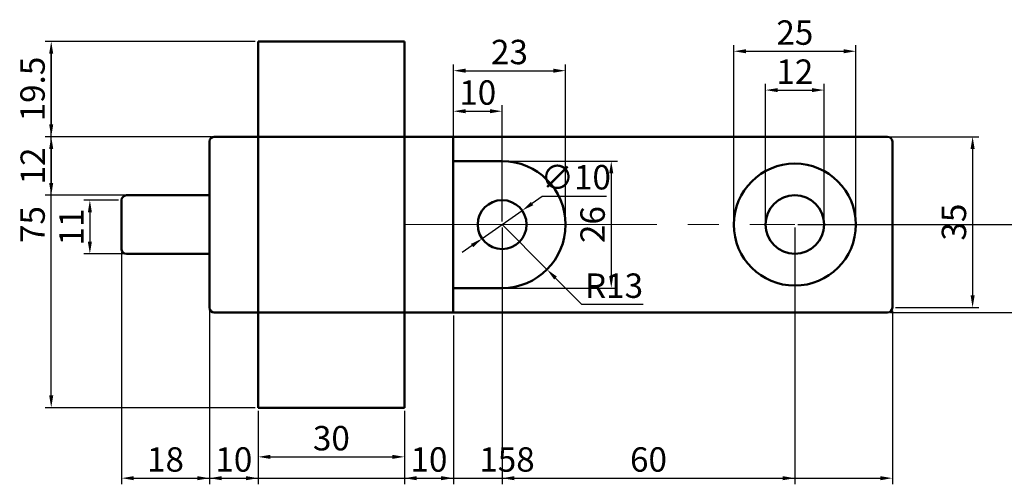
# Model space of a CAD drawing. Units: millimetres. Extents: x 2010 to 2347, y 1200 to 1429.
# Tile 1 of 3: x 2010 to 2212, y 1200 to 1295. Entities that reach past the tile are written whole.
import ezdxf

# ---------------------------------------------------------------- set-up
doc = ezdxf.new("R2010")
doc.units = ezdxf.units.MM
doc.linetypes.add('CENTER', pattern=[50.8, 31.75, -6.35, 6.35, -6.35])
for name, color, linetype, lineweight in [('M-CNTR', 4, 'CENTER', 18), ('M-DIMS', 2, 'Continuous', 25), ('M-OUTL', 7, 'Continuous', 50)]:
    doc.layers.add(name, color=color, linetype=linetype, lineweight=lineweight)
doc.styles.get("Standard").update_dxf_attribs({"font": 'arial.ttf'})
doc.dimstyles.new('ISO-25', dxfattribs={"dimtxt": 5, "dimasz": 2.5, "dimexe": 1.25, "dimexo": 0.625, "dimtad": 1, "dimtoh": 1, "dimdec": 0, "dimtxsty": 'Standard', "dimcen": 2.5, "dimadec": 0, "dimazin": 0, "dimtfac": 1, "dimtdec": 0, "dimtmove": 0, "dimatfit": 3, "dimfxl": 1, "dimarcsym": 0})

# ---------------------------------------------------------------- blocks, each defined once
blk = doc.blocks.new('*D9')
at = {"layer": 'Defpoints', "color": 0, "transparency": 16777216}
for p in [(2031.36, 1258.22), (2024.85, 1247.22), (2032.36, 1247.22)]:
    blk.add_point(p, dxfattribs=at)
at = {"layer": 'M-DIMS', "color": 0, "lineweight": -2, "transparency": 16777216}
for p, q in [((2030.73, 1258.22), (2023.6, 1258.22)), ((2024.85, 1255.72), (2024.85, 1249.72)), ((2031.73, 1247.22), (2023.6, 1247.22))]:
    blk.add_line(p, q, dxfattribs=at)
at = {"layer": 'M-DIMS', "color": 0, "transparency": 16777216}
for points in [[(2024.44, 1255.72), (2025.27, 1255.72), (2024.85, 1258.22)], [(2024.44, 1249.72), (2025.27, 1249.72), (2024.85, 1247.22)]]:
    blk.add_solid(points, dxfattribs=at)
at = {"layer": 'M-DIMS', "color": 0, "transparency": 16777216, "insert": (2021.72, 1252.72), "char_height": 5, "attachment_point": 5, "rotation": 90}
blk.add_mtext('11', dxfattribs=at)
blk = doc.blocks.new('*D10')
at = {"layer": 'Defpoints', "color": 0, "transparency": 16777216}
for p in [(2059.36, 1215.72), (2089.36, 1215.72), (2089.36, 1205.65)]:
    blk.add_point(p, dxfattribs=at)
at = {"layer": 'M-DIMS', "color": 0, "lineweight": -2, "transparency": 16777216}
for p, q in [((2059.36, 1215.09), (2059.36, 1204.4)), ((2089.36, 1215.09), (2089.36, 1204.4)), ((2061.86, 1205.65), (2086.86, 1205.65))]:
    blk.add_line(p, q, dxfattribs=at)
at = {"layer": 'M-DIMS', "color": 0, "transparency": 16777216}
for points in [[(2061.86, 1206.07), (2061.86, 1205.24), (2059.36, 1205.65)], [(2086.86, 1206.07), (2086.86, 1205.24), (2089.36, 1205.65)]]:
    blk.add_solid(points, dxfattribs=at)
at = {"layer": 'M-DIMS', "color": 0, "transparency": 16777216, "insert": (2074.36, 1208.83), "char_height": 5, "attachment_point": 5}
blk.add_mtext('30', dxfattribs=at)
blk = doc.blocks.new('*D11')
at = {"layer": 'Defpoints', "color": 0, "transparency": 16777216}
for p in [(2109.36, 1276.43), (2099.36, 1253.22), (2109.36, 1253.22)]:
    blk.add_point(p, dxfattribs=at)
at = {"layer": 'M-DIMS', "color": 0, "lineweight": -2, "transparency": 16777216}
for p, q in [((2099.36, 1253.84), (2099.36, 1277.68)), ((2109.36, 1253.84), (2109.36, 1277.68)), ((2101.86, 1276.43), (2106.86, 1276.43))]:
    blk.add_line(p, q, dxfattribs=at)
at = {"layer": 'M-DIMS', "color": 0, "transparency": 16777216}
for points in [[(2101.86, 1276.85), (2101.86, 1276.02), (2099.36, 1276.43)], [(2106.86, 1276.85), (2106.86, 1276.02), (2109.36, 1276.43)]]:
    blk.add_solid(points, dxfattribs=at)
at = {"layer": 'M-DIMS', "color": 0, "transparency": 16777216, "insert": (2104.36, 1279.61), "char_height": 5, "attachment_point": 5}
blk.add_mtext('10', dxfattribs=at)
blk = doc.blocks.new('*D12')
at = {"layer": 'Defpoints', "color": 0, "transparency": 16777216}
for p in [(2122.36, 1284.73), (2099.36, 1253.22), (2122.36, 1253.22)]:
    blk.add_point(p, dxfattribs=at)
at = {"layer": 'M-DIMS', "color": 0, "lineweight": -2, "transparency": 16777216}
for p, q in [((2099.36, 1253.84), (2099.36, 1285.98)), ((2122.36, 1253.84), (2122.36, 1285.98)), ((2101.86, 1284.73), (2119.86, 1284.73))]:
    blk.add_line(p, q, dxfattribs=at)
at = {"layer": 'M-DIMS', "color": 0, "transparency": 16777216}
for points in [[(2101.86, 1285.15), (2101.86, 1284.32), (2099.36, 1284.73)], [(2119.86, 1285.15), (2119.86, 1284.32), (2122.36, 1284.73)]]:
    blk.add_solid(points, dxfattribs=at)
at = {"layer": 'M-DIMS', "color": 0, "transparency": 16777216, "insert": (2110.86, 1287.91), "char_height": 5, "attachment_point": 5}
blk.add_mtext('23', dxfattribs=at)
blk = doc.blocks.new('*D13')
at = {"layer": 'Defpoints', "color": 0, "transparency": 16777216}
for p in [(2099.36, 1266.22), (2099.36, 1240.22), (2131.73, 1240.22)]:
    blk.add_point(p, dxfattribs=at)
at = {"layer": 'M-DIMS', "color": 0, "lineweight": -2, "transparency": 16777216}
for p, q in [((2099.98, 1266.22), (2132.98, 1266.22)), ((2131.73, 1263.72), (2131.73, 1242.72)), ((2099.98, 1240.22), (2132.98, 1240.22))]:
    blk.add_line(p, q, dxfattribs=at)
at = {"layer": 'M-DIMS', "color": 0, "transparency": 16777216}
for points in [[(2131.31, 1263.72), (2132.14, 1263.72), (2131.73, 1266.22)], [(2131.31, 1242.72), (2132.14, 1242.72), (2131.73, 1240.22)]]:
    blk.add_solid(points, dxfattribs=at)
at = {"layer": 'M-DIMS', "color": 0, "transparency": 16777216, "insert": (2128.55, 1253.22), "char_height": 5, "attachment_point": 5, "rotation": 90}
blk.add_mtext('26', dxfattribs=at)
blk = doc.blocks.new('*D14')
at = {"layer": 'Defpoints', "color": 0, "transparency": 16777216}
for p in [(2175.36, 1280.76), (2163.36, 1253.22), (2175.36, 1253.22)]:
    blk.add_point(p, dxfattribs=at)
at = {"layer": 'M-DIMS', "color": 0, "lineweight": -2, "transparency": 16777216}
for p, q in [((2163.36, 1253.84), (2163.36, 1282.01)), ((2175.36, 1253.84), (2175.36, 1282.01)), ((2165.86, 1280.76), (2172.86, 1280.76))]:
    blk.add_line(p, q, dxfattribs=at)
at = {"layer": 'M-DIMS', "color": 0, "transparency": 16777216}
for points in [[(2165.86, 1281.17), (2165.86, 1280.34), (2163.36, 1280.76)], [(2172.86, 1281.17), (2172.86, 1280.34), (2175.36, 1280.76)]]:
    blk.add_solid(points, dxfattribs=at)
at = {"layer": 'M-DIMS', "color": 0, "transparency": 16777216, "insert": (2169.36, 1283.89), "char_height": 5, "attachment_point": 5}
blk.add_mtext('12', dxfattribs=at)
blk = doc.blocks.new('*D15')
at = {"layer": 'Defpoints', "color": 0, "transparency": 16777216}
for p in [(2181.86, 1288.71), (2156.86, 1253.22), (2181.86, 1253.22)]:
    blk.add_point(p, dxfattribs=at)
at = {"layer": 'M-DIMS', "color": 0, "lineweight": -2, "transparency": 16777216}
for p, q in [((2156.86, 1253.84), (2156.86, 1289.96)), ((2181.86, 1253.84), (2181.86, 1289.96)), ((2159.36, 1288.71), (2179.36, 1288.71))]:
    blk.add_line(p, q, dxfattribs=at)
at = {"layer": 'M-DIMS', "color": 0, "transparency": 16777216}
for points in [[(2159.36, 1289.13), (2159.36, 1288.29), (2156.86, 1288.71)], [(2179.36, 1289.13), (2179.36, 1288.29), (2181.86, 1288.71)]]:
    blk.add_solid(points, dxfattribs=at)
at = {"layer": 'M-DIMS', "color": 0, "transparency": 16777216, "insert": (2169.36, 1291.89), "char_height": 5, "attachment_point": 5}
blk.add_mtext('25', dxfattribs=at)
blk = doc.blocks.new('*D16')
at = {"layer": 'Defpoints', "color": 0, "transparency": 16777216}
for p in [(2188.36, 1271.22), (2189.36, 1236.22), (2205.8, 1236.22)]:
    blk.add_point(p, dxfattribs=at)
at = {"layer": 'M-DIMS', "color": 0, "lineweight": -2, "transparency": 16777216}
for p, q in [((2188.98, 1271.22), (2207.05, 1271.22)), ((2205.8, 1268.72), (2205.8, 1238.72)), ((2189.98, 1236.22), (2207.05, 1236.22))]:
    blk.add_line(p, q, dxfattribs=at)
at = {"layer": 'M-DIMS', "color": 0, "transparency": 16777216}
for points in [[(2205.39, 1268.72), (2206.22, 1268.72), (2205.8, 1271.22)], [(2205.39, 1238.72), (2206.22, 1238.72), (2205.8, 1236.22)]]:
    blk.add_solid(points, dxfattribs=at)
at = {"layer": 'M-DIMS', "color": 0, "transparency": 16777216, "insert": (2202.62, 1253.72), "char_height": 5, "attachment_point": 5, "rotation": 90}
blk.add_mtext('35', dxfattribs=at)
blk = doc.blocks.new('*D23')
at = {"layer": 'Defpoints', "color": 0, "transparency": 16777216}
for p in [(2031.36, 1248.22), (2189.36, 1236.22), (2189.36, 1201.29)]:
    blk.add_point(p, dxfattribs=at)
at = {"layer": 'M-DIMS', "color": 0, "lineweight": -2, "transparency": 16777216}
for p, q in [((2031.36, 1247.59), (2031.36, 1200.04)), ((2189.36, 1235.59), (2189.36, 1200.04)), ((2033.86, 1201.29), (2186.86, 1201.29))]:
    blk.add_line(p, q, dxfattribs=at)
at = {"layer": 'M-DIMS', "color": 0, "transparency": 16777216}
for points in [[(2033.86, 1201.7), (2033.86, 1200.87), (2031.36, 1201.29)], [(2186.86, 1201.7), (2186.86, 1200.87), (2189.36, 1201.29)]]:
    blk.add_solid(points, dxfattribs=at)
at = {"layer": 'M-DIMS', "color": 0, "transparency": 16777216, "insert": (2110.36, 1204.47), "char_height": 5, "attachment_point": 5}
blk.add_mtext('158', dxfattribs=at)
blk = doc.blocks.new('*D24')
at = {"layer": 'Defpoints', "color": 0, "transparency": 16777216}
for p in [(2016.93, 1290.72), (2059.36, 1290.72), (2059.36, 1215.72)]:
    blk.add_point(p, dxfattribs=at)
at = {"layer": 'M-DIMS', "color": 0, "lineweight": -2, "transparency": 16777216}
for p, q in [((2058.73, 1290.72), (2015.68, 1290.72)), ((2016.93, 1218.22), (2016.93, 1288.22)), ((2058.73, 1215.72), (2015.68, 1215.72))]:
    blk.add_line(p, q, dxfattribs=at)
at = {"layer": 'M-DIMS', "color": 0, "transparency": 16777216}
for points in [[(2016.51, 1288.22), (2017.34, 1288.22), (2016.93, 1290.72)], [(2016.51, 1218.22), (2017.34, 1218.22), (2016.93, 1215.72)]]:
    blk.add_solid(points, dxfattribs=at)
at = {"layer": 'M-DIMS', "color": 0, "transparency": 16777216, "insert": (2013.76, 1253.22), "char_height": 5, "attachment_point": 5, "rotation": 90}
blk.add_mtext('75', dxfattribs=at)
blk = doc.blocks.new('*D27')
at = {"layer": 'Defpoints', "color": 0, "transparency": 16777216}
for p in [(2109.36, 1253.22), (2169.36, 1253.22), (2169.36, 1201.29)]:
    blk.add_point(p, dxfattribs=at)
at = {"layer": 'M-DIMS', "color": 0, "lineweight": -2, "transparency": 16777216}
for p, q in [((2109.36, 1252.59), (2109.36, 1200.04)), ((2169.36, 1252.59), (2169.36, 1200.04)), ((2111.86, 1201.29), (2166.86, 1201.29))]:
    blk.add_line(p, q, dxfattribs=at)
at = {"layer": 'M-DIMS', "color": 0, "transparency": 16777216}
for points in [[(2111.86, 1201.7), (2111.86, 1200.87), (2109.36, 1201.29)], [(2166.86, 1201.7), (2166.86, 1200.87), (2169.36, 1201.29)]]:
    blk.add_solid(points, dxfattribs=at)
at = {"layer": 'M-DIMS', "color": 0, "transparency": 16777216, "insert": (2139.36, 1204.47), "char_height": 5, "attachment_point": 5}
blk.add_mtext('60', dxfattribs=at)
blk = doc.blocks.new('*D33')
at = {"layer": 'Defpoints', "color": 0, "transparency": 16777216}
for p in [(2031.36, 1248.22), (2049.36, 1236.22), (2049.36, 1201.29)]:
    blk.add_point(p, dxfattribs=at)
at = {"layer": 'M-DIMS', "color": 0, "lineweight": -2, "transparency": 16777216}
for p, q in [((2031.36, 1247.59), (2031.36, 1200.04)), ((2049.36, 1235.59), (2049.36, 1200.04)), ((2033.86, 1201.29), (2046.86, 1201.29))]:
    blk.add_line(p, q, dxfattribs=at)
at = {"layer": 'M-DIMS', "color": 0, "transparency": 16777216}
for points in [[(2033.86, 1201.7), (2033.86, 1200.87), (2031.36, 1201.29)], [(2046.86, 1201.7), (2046.86, 1200.87), (2049.36, 1201.29)]]:
    blk.add_solid(points, dxfattribs=at)
at = {"layer": 'M-DIMS', "color": 0, "transparency": 16777216, "insert": (2040.36, 1204.47), "char_height": 5, "attachment_point": 5}
blk.add_mtext('18', dxfattribs=at)
blk = doc.blocks.new('*D34')
at = {"layer": 'Defpoints', "color": 0, "transparency": 16777216}
for p in [(2099.36, 1235.22), (2089.36, 1215.72), (2099.36, 1201.29)]:
    blk.add_point(p, dxfattribs=at)
at = {"layer": 'M-DIMS', "color": 0, "lineweight": -2, "transparency": 16777216}
for p, q in [((2099.36, 1234.59), (2099.36, 1200.04)), ((2089.36, 1215.09), (2089.36, 1200.04)), ((2091.86, 1201.29), (2096.86, 1201.29))]:
    blk.add_line(p, q, dxfattribs=at)
at = {"layer": 'M-DIMS', "color": 0, "transparency": 16777216}
for points in [[(2091.86, 1201.7), (2091.86, 1200.87), (2089.36, 1201.29)], [(2096.86, 1201.7), (2096.86, 1200.87), (2099.36, 1201.29)]]:
    blk.add_solid(points, dxfattribs=at)
at = {"layer": 'M-DIMS', "color": 0, "transparency": 16777216, "insert": (2094.36, 1204.47), "char_height": 5, "attachment_point": 5}
blk.add_mtext('10', dxfattribs=at)
blk = doc.blocks.new('*D35')
at = {"layer": 'Defpoints', "color": 0, "transparency": 16777216}
for p in [(2049.36, 1236.22), (2059.36, 1215.72), (2059.36, 1201.29)]:
    blk.add_point(p, dxfattribs=at)
at = {"layer": 'M-DIMS', "color": 0, "lineweight": -2, "transparency": 16777216}
for p, q in [((2049.36, 1235.59), (2049.36, 1200.04)), ((2059.36, 1215.09), (2059.36, 1200.04)), ((2051.86, 1201.29), (2056.86, 1201.29))]:
    blk.add_line(p, q, dxfattribs=at)
at = {"layer": 'M-DIMS', "color": 0, "transparency": 16777216}
for points in [[(2051.86, 1201.7), (2051.86, 1200.87), (2049.36, 1201.29)], [(2056.86, 1201.7), (2056.86, 1200.87), (2059.36, 1201.29)]]:
    blk.add_solid(points, dxfattribs=at)
at = {"layer": 'M-DIMS', "color": 0, "transparency": 16777216, "insert": (2054.36, 1204.47), "char_height": 5, "attachment_point": 5}
blk.add_mtext('10', dxfattribs=at)
blk = doc.blocks.new('*D43')
at = {"layer": 'Defpoints', "color": 0, "transparency": 16777216}
for p in [(2169.36, 1253.22), (2188.36, 1235.22), (2329.76, 1235.22)]:
    blk.add_point(p, dxfattribs=at)
at = {"layer": 'M-DIMS', "color": 0, "lineweight": -2, "transparency": 16777216}
for p, q in [((2169.98, 1253.22), (2331.01, 1253.22)), ((2329.76, 1250.72), (2329.76, 1237.72)), ((2188.98, 1235.22), (2331.01, 1235.22))]:
    blk.add_line(p, q, dxfattribs=at)
at = {"layer": 'M-DIMS', "color": 0, "transparency": 16777216}
for points in [[(2329.35, 1250.72), (2330.18, 1250.72), (2329.76, 1253.22)], [(2329.35, 1237.72), (2330.18, 1237.72), (2329.76, 1235.22)]]:
    blk.add_solid(points, dxfattribs=at)
at = {"layer": 'M-DIMS', "color": 0, "transparency": 16777216, "insert": (2326.58, 1244.22), "char_height": 5, "attachment_point": 5, "rotation": 90}
blk.add_mtext('18', dxfattribs=at)
blk = doc.blocks.new('*D46')
at = {"layer": 'Defpoints', "color": 0, "transparency": 16777216}
for p in [(2059.36, 1290.72), (2016.93, 1271.22), (2050.36, 1271.22)]:
    blk.add_point(p, dxfattribs=at)
at = {"layer": 'M-DIMS', "color": 0, "lineweight": -2, "transparency": 16777216}
for p, q in [((2058.73, 1290.72), (2015.68, 1290.72)), ((2016.93, 1288.22), (2016.93, 1273.72)), ((2049.73, 1271.22), (2015.68, 1271.22))]:
    blk.add_line(p, q, dxfattribs=at)
at = {"layer": 'M-DIMS', "color": 0, "transparency": 16777216}
for points in [[(2016.51, 1288.22), (2017.34, 1288.22), (2016.93, 1290.72)], [(2016.51, 1273.72), (2017.34, 1273.72), (2016.93, 1271.22)]]:
    blk.add_solid(points, dxfattribs=at)
at = {"layer": 'M-DIMS', "color": 0, "transparency": 16777216, "insert": (2013.75, 1280.97), "char_height": 5, "attachment_point": 5, "rotation": 90}
blk.add_mtext('19.5', dxfattribs=at)
blk = doc.blocks.new('*D47')
at = {"layer": 'Defpoints', "color": 0, "transparency": 16777216}
for p in [(2050.36, 1271.22), (2016.93, 1259.22), (2049.36, 1259.22)]:
    blk.add_point(p, dxfattribs=at)
at = {"layer": 'M-DIMS', "color": 0, "lineweight": -2, "transparency": 16777216}
for p, q in [((2049.73, 1271.22), (2015.68, 1271.22)), ((2016.93, 1268.72), (2016.93, 1261.72)), ((2048.73, 1259.22), (2015.68, 1259.22))]:
    blk.add_line(p, q, dxfattribs=at)
at = {"layer": 'M-DIMS', "color": 0, "transparency": 16777216}
for points in [[(2016.51, 1268.72), (2017.34, 1268.72), (2016.93, 1271.22)], [(2016.51, 1261.72), (2017.34, 1261.72), (2016.93, 1259.22)]]:
    blk.add_solid(points, dxfattribs=at)
at = {"layer": 'M-DIMS', "color": 0, "transparency": 16777216, "insert": (2013.79, 1265.22), "char_height": 5, "attachment_point": 5, "rotation": 90}
blk.add_mtext('12', dxfattribs=at)
blk = doc.blocks.new('*D49')
at = {"layer": 'Defpoints', "color": 0, "transparency": 16777216}
for p in [(2113.45, 1256.09), (2105.26, 1250.35)]:
    blk.add_point(p, dxfattribs=at)
at = {"layer": 'M-DIMS', "color": 0, "lineweight": -2, "transparency": 16777216}
for p, q in [((2117.55, 1258.95), (2115.5, 1257.52)), ((2130.76, 1258.95), (2117.55, 1258.95)), ((2105.26, 1250.35), (2113.45, 1256.09)), ((2103.21, 1248.92), (2101.16, 1247.48))]:
    blk.add_line(p, q, dxfattribs=at)
at = {"layer": 'M-DIMS', "color": 0, "transparency": 16777216}
for points in [[(2115.26, 1257.86), (2115.74, 1257.18), (2113.45, 1256.09)], [(2102.97, 1249.26), (2103.45, 1248.57), (2105.26, 1250.35)]]:
    blk.add_solid(points, dxfattribs=at)
at = {"layer": 'M-DIMS', "color": 0, "transparency": 16777216, "insert": (2124.46, 1262.27), "char_height": 5, "attachment_point": 5}
blk.add_mtext('∅10', dxfattribs=at)
blk = doc.blocks.new('*D50')
at = {"layer": 'Defpoints', "color": 0, "transparency": 16777216}
for p in [(2109.36, 1253.22), (2118.55, 1244.03)]:
    blk.add_point(p, dxfattribs=at)
at = {"layer": 'M-DIMS', "color": 0, "lineweight": -2, "transparency": 16777216}
for p, q in [((2109.36, 1253.22), (2118.55, 1244.03)), ((2125.7, 1236.88), (2120.32, 1242.26)), ((2138.27, 1236.88), (2125.7, 1236.88))]:
    blk.add_line(p, q, dxfattribs=at)
at = {"layer": 'M-DIMS', "color": 0, "transparency": 16777216}
blk.add_solid([(2120.61, 1242.56), (2120.03, 1241.97), (2118.55, 1244.03)], dxfattribs=at)
at = {"layer": 'M-DIMS', "color": 0, "transparency": 16777216, "insert": (2132.3, 1240.06), "char_height": 5, "attachment_point": 5}
blk.add_mtext('R13', dxfattribs=at)

msp = doc.modelspace()

# ---------------------------------------------------------------- linework, layer by layer
at = {"layer": 'M-CNTR'}
for p, q in [((2089.3551, 1253.2177), (2099.3551, 1253.2177)), ((2099.3551, 1253.2177), (2096.9629, 1253.2177)), ((2099.3551, 1253.2177), (2096.9629, 1253.2177)), ((2099.3551, 1253.2177), (2109.3551, 1253.2177)), ((2109.3551, 1253.2177), (2169.3551, 1253.2177))]:
    msp.add_line(p, q, dxfattribs=at)
at = {"layer": 'M-OUTL'}
for p, q in [((2059.3551, 1271.2177), (2059.3551, 1290.7177)), ((2059.3551, 1290.7177), (2089.3551, 1290.7177)), ((2089.3551, 1290.7177), (2089.3551, 1215.7177)), ((2049.3551, 1270.2177), (2049.3551, 1236.2177)), ((2188.3551, 1271.2177), (2050.3551, 1271.2177)), ((2050.3551, 1271.2177), (2059.3551, 1271.2177)), ((2059.3551, 1215.7177), (2059.3551, 1271.2177)), ((2099.3551, 1253.2177), (2099.3551, 1271.2177)), ((2099.3551, 1271.2177), (2099.3551, 1266.2177)), ((2189.3551, 1236.2177), (2189.3551, 1270.2177)), ((2099.3551, 1266.2177), (2109.3551, 1266.2177)), ((2031.3551, 1258.2177), (2031.3551, 1248.2177)), ((2049.3551, 1259.2177), (2032.3551, 1259.2177)), ((2049.3551, 1253.2177), (2049.3551, 1259.2177)), ((2099.3551, 1253.2177), (2099.3551, 1235.2177)), ((2032.3551, 1247.2177), (2049.3551, 1247.2177)), ((2099.3551, 1235.2177), (2099.3551, 1240.2177)), ((2099.3551, 1240.2177), (2109.3551, 1240.2177)), ((2050.3551, 1235.2177), (2188.3551, 1235.2177)), ((2089.3551, 1215.7177), (2059.3551, 1215.7177))]:
    msp.add_line(p, q, dxfattribs=at)
for centre, radius in [((2169.3551, 1253.2177), 12.5), ((2109.3551, 1253.2177), 5), ((2169.3551, 1253.2177), 6)]:
    msp.add_circle(centre, radius, dxfattribs=at)
for centre, radius, start, end in [((2050.3551, 1270.2177), 1, 90, 180), ((2188.3551, 1270.2177), 1, 0, 90), ((2109.3551, 1253.2177), 13, 270, 90), ((2032.3551, 1258.2177), 1, 90, 180), ((2032.3551, 1248.2177), 1, 180, 270), ((2050.3551, 1236.2177), 1, 180, 270), ((2188.3551, 1236.2177), 1, 270, 0)]:
    msp.add_arc(centre, radius, start, end, dxfattribs=at)

# ---------------------------------------------------------------- dimensions: what is measured, and where the dimension line sits
at = {"layer": 'M-DIMS'}
for base, p1, p2, override, picture, middle in [((2181.8551, 1288.7113), (2156.8551, 1253.2177), (2181.8551, 1253.2177), {"dimclrd": 0, "dimclre": 0, "dimclrt": 0}, '*D15', (2169.3551, 1291.8892)), ((2122.3551, 1284.7341), (2099.3551, 1253.2177), (2122.3551, 1253.2177), {"dimclrd": 0, "dimclre": 0, "dimclrt": 0}, '*D12', (2110.8551, 1287.9137)), ((2175.3551, 1280.757), (2163.3551, 1253.2177), (2175.3551, 1253.2177), {"dimclrd": 0, "dimclre": 0, "dimclrt": 0}, '*D14', (2169.3551, 1283.8922)), ((2109.3551, 1276.4339), (2099.3551, 1253.2177), (2109.3551, 1253.2177), {"dimclrd": 0, "dimclre": 0, "dimclrt": 0}, '*D11', (2104.3551, 1279.6118)), ((2169.3551, 1201.2877), (2109.3551, 1253.2177), (2169.3551, 1253.2177), {"dimdec": 0, "dimlfac": 1, "dimrnd": 0, "dimzin": 0, "dimdsep": 46, "dimlunit": 2}, '*D27', (2139.3551, 1204.4655)), ((2189.3551, 1201.2877), (2031.3551, 1248.2177), (2189.3551, 1236.2177), {"dimdec": 0, "dimlfac": 1, "dimrnd": 0, "dimzin": 0, "dimdsep": 46, "dimlunit": 2}, '*D23', (2110.3551, 1204.4655)), ((2049.3551, 1201.2877), (2031.3551, 1248.2177), (2049.3551, 1236.2177), {"dimdec": 0, "dimlfac": 1, "dimrnd": 0, "dimzin": 0, "dimdsep": 46, "dimlunit": 2}, '*D33', (2040.3551, 1204.4655)), ((2059.3551, 1201.2877), (2049.3551, 1236.2177), (2059.3551, 1215.7177), {"dimdec": 0, "dimlfac": 1, "dimrnd": 0, "dimzin": 0, "dimdsep": 46, "dimlunit": 2}, '*D35', (2054.3551, 1204.4655)), ((2099.3551, 1201.2877), (2089.3551, 1215.7177), (2099.3551, 1235.2177), {"dimdec": 0, "dimlfac": 1, "dimrnd": 0, "dimzin": 0, "dimdsep": 46, "dimlunit": 2}, '*D34', (2094.3551, 1204.4655)), ((2089.3551, 1205.6537), (2059.3551, 1215.7177), (2089.3551, 1215.7177), {"dimclrd": 0, "dimclre": 0, "dimclrt": 0}, '*D10', (2074.3551, 1208.8333))]:
    dim = msp.add_linear_dim(base=base, p1=p1, p2=p2, dimstyle='ISO-25', override=override, dxfattribs=at)
    dim.commit()
    dim.dimension.update_dxf_attribs({"geometry": picture, "text_midpoint": middle})
for base, p1, p2, override, picture, middle in [((2016.9251, 1271.2177), (2059.3551, 1290.7177), (2050.3551, 1271.2177), {"dimdec": 1, "dimlfac": 1, "dimrnd": 0, "dimzin": 0, "dimdsep": 46, "dimlunit": 2}, '*D46', (2013.7472, 1280.9677)), ((2016.9251, 1290.7177), (2059.3551, 1215.7177), (2059.3551, 1290.7177), {"dimdec": 0, "dimlfac": 1, "dimrnd": 0, "dimzin": 0, "dimdsep": 46, "dimlunit": 2}, '*D24', (2013.7574, 1253.2177)), ((2016.9251, 1259.2177), (2050.3551, 1271.2177), (2049.3551, 1259.2177), {"dimdec": 0, "dimlfac": 1, "dimrnd": 0, "dimzin": 0, "dimdsep": 46, "dimlunit": 2}, '*D47', (2013.7899, 1265.2177)), ((2205.8024, 1236.2177), (2188.3551, 1271.2177), (2189.3551, 1236.2177), {"dimclrd": 0, "dimclre": 0, "dimclrt": 0}, '*D16', (2202.6228, 1253.7177)), ((2131.7273, 1240.2177), (2099.3551, 1266.2177), (2099.3551, 1240.2177), {"dimclrd": 0, "dimclre": 0, "dimclrt": 0}, '*D13', (2128.5495, 1253.2177)), ((2024.8536, 1247.2177), (2031.3551, 1258.2177), (2032.3551, 1247.2177), {"dimclrd": 0, "dimclre": 0, "dimclrt": 0}, '*D9', (2021.7184, 1252.7177)), ((2329.7618, 1235.2177), (2169.3551, 1253.2177), (2188.3551, 1235.2177), {"dimdec": 0, "dimlfac": 1, "dimrnd": 0, "dimzin": 0, "dimdsep": 46, "dimlunit": 2}, '*D43', (2326.5839, 1244.2177))]:
    dim = msp.add_linear_dim(base=base, p1=p1, p2=p2, angle=90, dimstyle='ISO-25', override=override, dxfattribs=at)
    dim.commit()
    dim.dimension.update_dxf_attribs({"geometry": picture, "text_midpoint": middle})
dim = msp.add_diameter_dim_2p(p1=(2105.2593, 1250.3498), p2=(2113.4508, 1256.0856), dimstyle='ISO-25', override={"dimdec": 0, "dimlfac": 1, "dimrnd": 0, "dimzin": 0, "dimdsep": 46, "dimlunit": 2}, dxfattribs=at)
dim.commit()
dim.dimension.update_dxf_attribs({"geometry": '*D49', "text_midpoint": (2124.4642, 1258.9535), "dimtype": 163})
dim = msp.add_radius_dim(center=(2109.3551, 1253.2177), mpoint=(2118.5511, 1244.0289), dimstyle='ISO-25', override={"dimdec": 0, "dimlfac": 1, "dimrnd": 0, "dimzin": 0, "dimdsep": 46, "dimlunit": 2}, dxfattribs=at)
dim.commit()
dim.dimension.update_dxf_attribs({"geometry": '*D50', "text_midpoint": (2132.3009, 1240.0631)})

doc.saveas('drawing.dxf')
